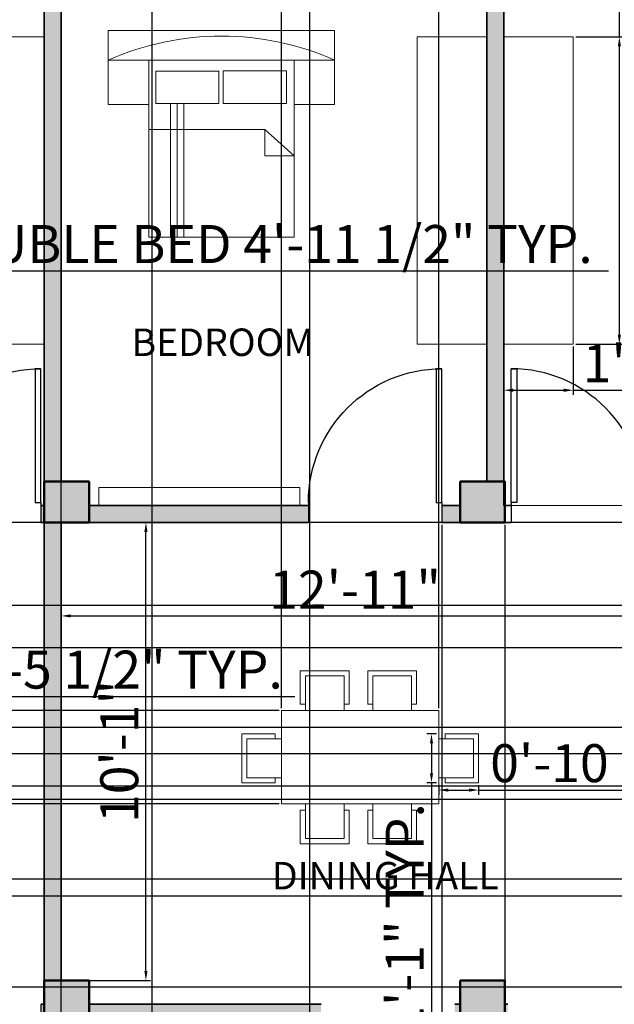
# Model space of a CAD drawing. Units: inches. Extents: x 2312 to 2808, y 1290 to 1909.
# Tile 3 of 5: x 2476 to 2633, y 1503 to 1763. Entities that reach past the tile are written whole.
import ezdxf

# ---------------------------------------------------------------- set-up
doc = ezdxf.new("R2010")
doc.units = ezdxf.units.IN
for name, color, linetype, lineweight in [('A-ANNO-DIMS', 2, 'Continuous', 18), ('A-AREA-IDEN', 7, 'Continuous', 25), ('A-COLS-PATT', 1, 'Continuous', 13), ('A-FLOR-CASE', 181, 'Continuous', 20), ('A-WALL-PATT', 150, 'Continuous', 13), ('COLUMN', 1, 'Continuous', 50), ('DOOR', 50, 'Continuous', 25), ('FUR', 130, 'Continuous', 18), ('WALL', 7, 'Continuous', 35)]:
    doc.layers.add(name, color=color, linetype=linetype, lineweight=lineweight)
doc.styles.get("Standard").update_dxf_attribs({"font": 'arial.ttf'})
doc.dimstyles.new('ISO-25', dxfattribs={"dimtxt": 10, "dimasz": 2.5, "dimexe": 1.25, "dimexo": 0.625, "dimtad": 1, "dimdec": 0, "dimlunit": 4, "dimtxsty": 'Standard', "dimcen": 2.5, "dimadec": 0, "dimazin": 0, "dimtfac": 1, "dimtdec": 0, "dimtmove": 0, "dimatfit": 3, "dimfxl": 1, "dimarcsym": 0})

# ---------------------------------------------------------------- blocks, each defined once
blk = doc.blocks.new('*U2')
for p, q in [((0, 0), (0, -6)), ((40, 0), (40, -6))]:
    blk.add_line(p, q)
blk.add_lwpolyline([(0, 0), (0, 40), (1.75, 40), (1.75, 0)], close=True)
blk.add_arc((0, 0), 40, 0, 90)
blk = doc.blocks.new('*D12')
at = {"layer": 'A-ANNO-DIMS', "color": 0, "lineweight": -2, "transparency": 16777216}
for p, q in [((2604.24, 1764.94), (2740.72, 1765.28)), ((2739.79, 1637.55), (2739.48, 1762.78)), ((2604.56, 1634.72), (2741.04, 1635.06))]:
    blk.add_line(p, q, dxfattribs=at)
at = {"layer": 'A-ANNO-DIMS', "color": 0, "transparency": 16777216}
for points in [[(2739.89, 1762.78), (2739.06, 1762.78), (2739.47, 1765.28)], [(2740.2, 1637.56), (2739.37, 1637.55), (2739.79, 1635.05)]]:
    blk.add_solid(points, dxfattribs=at)
at = {"layer": 'Defpoints', "color": 0, "transparency": 16777216}
for p in [(2603.61, 1764.94), (2739.47, 1765.28), (2603.93, 1634.72)]:
    blk.add_point(p, dxfattribs=at)
at = {"layer": 'A-ANNO-DIMS', "color": 0, "transparency": 16777216, "insert": (2745.36, 1700.18), "char_height": 10, "attachment_point": 5, "rotation": 270.1423}
blk.add_mtext('10\'-10"', dxfattribs=at)
blk = doc.blocks.new('*D22')
at = {"layer": 'A-ANNO-DIMS', "color": 0, "lineweight": -2, "transparency": 16777216}
for p, q in [((2486.93, 1629.59), (2486.93, 1604.33)), ((2641.91, 1629.59), (2641.91, 1604.33)), ((2489.43, 1605.58), (2639.41, 1605.58))]:
    blk.add_line(p, q, dxfattribs=at)
at = {"layer": 'A-ANNO-DIMS', "color": 0, "transparency": 16777216}
for points in [[(2489.43, 1606), (2489.43, 1605.17), (2486.93, 1605.58)], [(2639.41, 1606), (2639.41, 1605.17), (2641.91, 1605.58)]]:
    blk.add_solid(points, dxfattribs=at)
at = {"layer": 'Defpoints', "color": 0, "transparency": 16777216}
for p in [(2486.93, 1630.22), (2641.91, 1630.22), (2641.91, 1605.58)]:
    blk.add_point(p, dxfattribs=at)
at = {"layer": 'A-ANNO-DIMS', "color": 0, "transparency": 16777216, "insert": (2564.42, 1611.23), "char_height": 10, "attachment_point": 5}
blk.add_mtext('12\'-11"', dxfattribs=at)
blk = doc.blocks.new('*D23')
at = {"layer": 'A-ANNO-DIMS', "color": 0, "lineweight": -2, "transparency": 16777216}
for p, q in [((2487.56, 1630.22), (2510.52, 1630.22)), ((2509.27, 1511.99), (2509.27, 1627.72)), ((2487.56, 1509.49), (2510.52, 1509.49))]:
    blk.add_line(p, q, dxfattribs=at)
at = {"layer": 'A-ANNO-DIMS', "color": 0, "transparency": 16777216}
for points in [[(2508.85, 1627.72), (2509.69, 1627.72), (2509.27, 1630.22)], [(2508.85, 1511.99), (2509.69, 1511.99), (2509.27, 1509.49)]]:
    blk.add_solid(points, dxfattribs=at)
at = {"layer": 'Defpoints', "color": 0, "transparency": 16777216}
for p in [(2486.93, 1630.22), (2509.27, 1630.22), (2486.93, 1509.49)]:
    blk.add_point(p, dxfattribs=at)
at = {"layer": 'A-ANNO-DIMS', "color": 0, "transparency": 16777216, "insert": (2503.54, 1569.86), "char_height": 10, "attachment_point": 5, "rotation": 90}
blk.add_mtext('10\'-1"', dxfattribs=at)
blk = doc.blocks.new('BED-DOUBLE')
for p, q in [((0, 46.6), (0, 54.42)), ((0, 54.42), (59.67, 54.42)), ((59.67, 54.42), (59.67, 46.6)), ((16.43, 35.15), (16.43, 0)), ((18.15, 35.15), (18.15, 0)), ((19.9, 35.15), (19.9, 0)), ((10.68, 28.37), (10.68, 28.37)), ((10.68, 28.37), (41.23, 28.37)), ((41.23, 28.37), (41.23, 21.43)), ((48.99, 21.43), (41.23, 28.37)), ((41.23, 21.43), (48.99, 21.43))]:
    blk.add_line(p, q)
for points in [[(10.68, 46.6), (0, 46.6), (0, 34.89), (10.68, 34.89)], [(10.68, 46.6), (48.99, 46.6), (48.99, 0), (10.68, 0)], [(59.67, 46.6), (48.99, 46.6), (48.99, 34.89), (59.67, 34.89)], [(12.51, 43.74), (29.18, 43.74), (29.18, 35.15), (12.51, 35.15)], [(30.28, 43.78), (46.95, 43.78), (46.95, 35.19), (30.28, 35.19)]]:
    blk.add_lwpolyline(points, close=True)
blk.add_arc((29.84, -20.26), 73.22, 65.9516, 114.0484)
blk = doc.blocks.new('CHAIR-DINING')
for p, q in [((0, 1.67), (0, 10.49)), ((0, 10.49), (12.88, 10.49)), ((12.88, 10.49), (12.88, 1.67)), ((1.34, 1.67), (0, 1.67)), ((12.88, 1.67), (11.58, 1.67))]:
    blk.add_line(p, q)
blk.add_lwpolyline([(1.34, 0), (11.58, 0), (11.58, 9.15), (1.34, 9.15)], close=True)
blk = doc.blocks.new('BEDROOM-STORAGE')
blk.add_lwpolyline([(18.34, 80.97), (0, 80.97), (0, 0), (18.34, 0)], close=True)
blk = doc.blocks.new('BEDROOM-WALL-UNIT')
blk.add_lwpolyline([(0, 0), (52.94, 0), (52.94, 4.76), (0, 4.76)], close=True)
blk = doc.blocks.new('*D29')
at = {"layer": 'A-ANNO-DIMS', "color": 0, "lineweight": -2, "transparency": 16777216}
for p, q in [((2382.33, 1704.84), (2382.33, 1695.26)), ((2442, 1704.84), (2442, 1695.26)), ((2384.83, 1696.51), (2439.5, 1696.51)), ((2442, 1696.51), (2631.22, 1696.51))]:
    blk.add_line(p, q, dxfattribs=at)
at = {"layer": 'A-ANNO-DIMS', "color": 0, "transparency": 16777216}
for points in [[(2384.83, 1696.93), (2384.83, 1696.09), (2382.33, 1696.51)], [(2439.5, 1696.93), (2439.5, 1696.09), (2442, 1696.51)]]:
    blk.add_solid(points, dxfattribs=at)
at = {"layer": 'Defpoints', "color": 0, "transparency": 16777216}
for p in [(2382.33, 1705.46), (2442, 1705.46), (2442, 1696.51)]:
    blk.add_point(p, dxfattribs=at)
at = {"layer": 'A-ANNO-DIMS', "color": 0, "transparency": 16777216, "insert": (2537.86, 1702.31), "char_height": 10, "attachment_point": 5}
blk.add_mtext('DOUBLE BED 4\'-11 1/2" TYP.', dxfattribs=at)
blk = doc.blocks.new('*D31')
at = {"layer": 'A-ANNO-DIMS', "color": 0, "lineweight": -2, "transparency": 16777216}
for p, q in [((2634.1, 1758.19), (2634.1, 1909.46)), ((2622.58, 1758.19), (2635.35, 1758.19)), ((2634.1, 1679.72), (2634.1, 1755.69)), ((2622.58, 1677.22), (2635.35, 1677.22))]:
    blk.add_line(p, q, dxfattribs=at)
at = {"layer": 'A-ANNO-DIMS', "color": 0, "transparency": 16777216}
for points in [[(2633.68, 1755.69), (2634.51, 1755.69), (2634.1, 1758.19)], [(2633.68, 1679.72), (2634.51, 1679.72), (2634.1, 1677.22)]]:
    blk.add_solid(points, dxfattribs=at)
at = {"layer": 'Defpoints', "color": 0, "transparency": 16777216}
for p in [(2621.95, 1758.19), (2634.1, 1758.19), (2621.95, 1677.22)]:
    blk.add_point(p, dxfattribs=at)
at = {"layer": 'A-ANNO-DIMS', "color": 0, "transparency": 16777216, "insert": (2628.3, 1835.07), "char_height": 10, "attachment_point": 5, "rotation": 90}
blk.add_mtext('WARDROBE 6\'-9" TYP.', dxfattribs=at)
blk = doc.blocks.new('*D32')
at = {"layer": 'A-ANNO-DIMS', "color": 0, "lineweight": -2, "transparency": 16777216}
for p, q in [((2603.61, 1676.59), (2603.61, 1663.82)), ((2621.95, 1676.59), (2621.95, 1663.82)), ((2606.11, 1665.07), (2619.45, 1665.07)), ((2621.95, 1665.07), (2709.02, 1665.07))]:
    blk.add_line(p, q, dxfattribs=at)
at = {"layer": 'A-ANNO-DIMS', "color": 0, "transparency": 16777216}
for points in [[(2606.11, 1665.49), (2606.11, 1664.65), (2603.61, 1665.07)], [(2619.45, 1665.49), (2619.45, 1664.65), (2621.95, 1665.07)]]:
    blk.add_solid(points, dxfattribs=at)
at = {"layer": 'Defpoints', "color": 0, "transparency": 16777216}
for p in [(2603.61, 1677.22), (2621.95, 1677.22), (2621.95, 1665.07)]:
    blk.add_point(p, dxfattribs=at)
at = {"layer": 'A-ANNO-DIMS', "color": 0, "transparency": 16777216, "insert": (2666.73, 1670.87), "char_height": 10, "attachment_point": 5}
blk.add_mtext('1\'-6 1/2" TYP.', dxfattribs=at)
blk = doc.blocks.new('*D33')
at = {"layer": 'A-ANNO-DIMS', "color": 0, "lineweight": -2, "transparency": 16777216}
for p, q in [((2381.24, 1493.33), (2381.24, 1484.77)), ((2434.18, 1493.33), (2434.18, 1484.77)), ((2383.74, 1486.02), (2431.68, 1486.02)), ((2434.18, 1486.02), (2577.69, 1486.02))]:
    blk.add_line(p, q, dxfattribs=at)
at = {"layer": 'A-ANNO-DIMS', "color": 0, "transparency": 16777216}
for points in [[(2383.74, 1486.43), (2383.74, 1485.6), (2381.24, 1486.02)], [(2431.68, 1486.43), (2431.68, 1485.6), (2434.18, 1486.02)]]:
    blk.add_solid(points, dxfattribs=at)
at = {"layer": 'Defpoints', "color": 0, "transparency": 16777216}
for p in [(2381.24, 1493.96), (2434.18, 1493.96), (2434.18, 1486.02)]:
    blk.add_point(p, dxfattribs=at)
at = {"layer": 'A-ANNO-DIMS', "color": 0, "transparency": 16777216, "insert": (2507.19, 1491.73), "char_height": 10, "attachment_point": 5}
blk.add_mtext('WALL UNIT 4\'-5" TYP.', dxfattribs=at)
blk = doc.blocks.new('*D35')
at = {"layer": 'A-ANNO-DIMS', "color": 0, "lineweight": -2, "transparency": 16777216}
for p, q in [((2585.87, 1574.5), (2583.31, 1574.5)), ((2584.56, 1572), (2584.56, 1564.12)), ((2585.87, 1561.62), (2583.31, 1561.62)), ((2584.56, 1561.62), (2584.56, 1449.68))]:
    blk.add_line(p, q, dxfattribs=at)
at = {"layer": 'A-ANNO-DIMS', "color": 0, "transparency": 16777216}
for points in [[(2584.15, 1572), (2584.98, 1572), (2584.56, 1574.5)], [(2584.15, 1564.12), (2584.98, 1564.12), (2584.56, 1561.62)]]:
    blk.add_solid(points, dxfattribs=at)
at = {"layer": 'Defpoints', "color": 0, "transparency": 16777216}
for p in [(2586.49, 1574.5), (2584.56, 1561.62), (2586.49, 1561.62)]:
    blk.add_point(p, dxfattribs=at)
at = {"layer": 'A-ANNO-DIMS', "color": 0, "transparency": 16777216, "insert": (2578.77, 1504.4), "char_height": 10, "attachment_point": 5, "rotation": 90}
blk.add_mtext('CHAIR 1\'-1" TYP.', dxfattribs=at)
blk = doc.blocks.new('*D36')
at = {"layer": 'A-ANNO-DIMS', "color": 0, "lineweight": -2, "transparency": 16777216}
for p, q in [((2586.49, 1560.99), (2586.49, 1558.44)), ((2596.99, 1560.99), (2596.99, 1558.44)), ((2588.99, 1559.69), (2594.49, 1559.69)), ((2596.99, 1559.69), (2692.76, 1559.69))]:
    blk.add_line(p, q, dxfattribs=at)
at = {"layer": 'A-ANNO-DIMS', "color": 0, "transparency": 16777216}
for points in [[(2588.99, 1560.1), (2588.99, 1559.27), (2586.49, 1559.69)], [(2594.49, 1560.1), (2594.49, 1559.27), (2596.99, 1559.69)]]:
    blk.add_solid(points, dxfattribs=at)
at = {"layer": 'Defpoints', "color": 0, "transparency": 16777216}
for p in [(2586.49, 1561.62), (2596.99, 1561.62), (2596.99, 1559.69)]:
    blk.add_point(p, dxfattribs=at)
at = {"layer": 'A-ANNO-DIMS', "color": 0, "transparency": 16777216, "insert": (2646.12, 1565.48), "char_height": 10, "attachment_point": 5}
blk.add_mtext('0\'-10 1/2" TYP.', dxfattribs=at)
blk = doc.blocks.new('*D37')
at = {"layer": 'A-ANNO-DIMS', "color": 0, "lineweight": -2, "transparency": 16777216}
for p, q in [((2380.65, 1586.33), (2380.65, 1583.1)), ((2398.06, 1586.33), (2398.06, 1583.1)), ((2383.15, 1584.35), (2395.56, 1584.35)), ((2398.06, 1584.35), (2548.49, 1584.35))]:
    blk.add_line(p, q, dxfattribs=at)
at = {"layer": 'A-ANNO-DIMS', "color": 0, "transparency": 16777216}
for points in [[(2383.15, 1584.76), (2383.15, 1583.93), (2380.65, 1584.35)], [(2395.56, 1584.76), (2395.56, 1583.93), (2398.06, 1584.35)]]:
    blk.add_solid(points, dxfattribs=at)
at = {"layer": 'Defpoints', "color": 0, "transparency": 16777216}
for p in [(2380.65, 1586.96), (2398.06, 1586.96), (2398.06, 1584.35)]:
    blk.add_point(p, dxfattribs=at)
at = {"layer": 'A-ANNO-DIMS', "color": 0, "transparency": 16777216, "insert": (2474.53, 1590.14), "char_height": 10, "attachment_point": 5}
blk.add_mtext('BURNER 1\'-5 1/2" TYP.', dxfattribs=at)
blk = doc.blocks.new('*D41')
at = {"layer": 'A-ANNO-DIMS', "color": 0, "lineweight": -2, "transparency": 16777216}
for p, q in [((2443.93, 1546.83), (2443.93, 1804.57)), ((2482.43, 1510.12), (2482.43, 1804.57)), ((2446.43, 1803.32), (2479.93, 1803.32)), ((2482.43, 1803.32), (2536.06, 1803.32))]:
    blk.add_line(p, q, dxfattribs=at)
at = {"layer": 'A-ANNO-DIMS', "color": 0, "transparency": 16777216}
for points in [[(2446.43, 1803.73), (2446.43, 1802.9), (2443.93, 1803.32)], [(2479.93, 1803.73), (2479.93, 1802.9), (2482.43, 1803.32)]]:
    blk.add_solid(points, dxfattribs=at)
at = {"layer": 'Defpoints', "color": 0, "transparency": 16777216}
for p in [(2482.43, 1803.32), (2443.93, 1546.2), (2482.43, 1509.49)]:
    blk.add_point(p, dxfattribs=at)
at = {"layer": 'A-ANNO-DIMS', "color": 0, "transparency": 16777216, "insert": (2510.5, 1809.12), "char_height": 10, "attachment_point": 5}
blk.add_mtext('3\'-2 1/2"', dxfattribs=at)
blk = doc.blocks.new('*D43')
at = {"layer": 'A-ANNO-DIMS', "color": 0, "lineweight": -2, "transparency": 16777216}
for p, q in [((2486.93, 1401.34), (2486.93, 1804.57)), ((2510.93, 1401.34), (2510.93, 1804.57)), ((2489.43, 1803.32), (2508.43, 1803.32)), ((2510.93, 1803.32), (2541.44, 1803.32))]:
    blk.add_line(p, q, dxfattribs=at)
at = {"layer": 'A-ANNO-DIMS', "color": 0, "transparency": 16777216}
for points in [[(2489.43, 1803.73), (2489.43, 1802.9), (2486.93, 1803.32)], [(2508.43, 1803.73), (2508.43, 1802.9), (2510.93, 1803.32)]]:
    blk.add_solid(points, dxfattribs=at)
at = {"layer": 'Defpoints', "color": 0, "transparency": 16777216}
for p in [(2510.93, 1803.32), (2486.93, 1400.72), (2510.93, 1400.72)]:
    blk.add_point(p, dxfattribs=at)
at = {"layer": 'A-ANNO-DIMS', "color": 0, "transparency": 16777216, "insert": (2527.44, 1809.05), "char_height": 10, "attachment_point": 5}
blk.add_mtext('2\'-0"', dxfattribs=at)
blk = doc.blocks.new('*D50')
at = {"layer": 'A-ANNO-DIMS', "color": 0, "lineweight": -2, "transparency": 16777216}
for p, q in [((2446.36, 1635.34), (2446.36, 1804.57)), ((2482.43, 1635.34), (2482.43, 1804.57)), ((2448.86, 1803.32), (2479.93, 1803.32))]:
    blk.add_line(p, q, dxfattribs=at)
at = {"layer": 'A-ANNO-DIMS', "color": 0, "transparency": 16777216}
for points in [[(2448.86, 1803.73), (2448.86, 1802.9), (2446.36, 1803.32)], [(2479.93, 1803.73), (2479.93, 1802.9), (2482.43, 1803.32)]]:
    blk.add_solid(points, dxfattribs=at)
at = {"layer": 'Defpoints', "color": 0, "transparency": 16777216}
for p in [(2482.43, 1803.32), (2446.36, 1634.72), (2482.43, 1634.72)]:
    blk.add_point(p, dxfattribs=at)
at = {"layer": 'A-ANNO-DIMS', "color": 0, "transparency": 16777216, "insert": (2464.4, 1809.05), "char_height": 10, "attachment_point": 5}
blk.add_mtext('3\'-0"', dxfattribs=at)
blk = doc.blocks.new('*D54')
at = {"layer": 'A-ANNO-DIMS', "color": 0, "lineweight": -2, "transparency": 16777216}
for p, q in [((2545.01, 1581.25), (2545.01, 1804.57)), ((2586.49, 1581.25), (2586.49, 1804.57)), ((2547.51, 1803.32), (2583.99, 1803.32)), ((2586.49, 1803.32), (2640.12, 1803.32))]:
    blk.add_line(p, q, dxfattribs=at)
at = {"layer": 'A-ANNO-DIMS', "color": 0, "transparency": 16777216}
for points in [[(2547.51, 1803.73), (2547.51, 1802.9), (2545.01, 1803.32)], [(2583.99, 1803.73), (2583.99, 1802.9), (2586.49, 1803.32)]]:
    blk.add_solid(points, dxfattribs=at)
at = {"layer": 'Defpoints', "color": 0, "transparency": 16777216}
for p in [(2586.49, 1803.32), (2545.01, 1580.62), (2586.49, 1580.62)]:
    blk.add_point(p, dxfattribs=at)
at = {"layer": 'A-ANNO-DIMS', "color": 0, "transparency": 16777216, "insert": (2614.56, 1809.12), "char_height": 10, "attachment_point": 5}
blk.add_mtext('3\'-5 1/2"', dxfattribs=at)
blk = doc.blocks.new('*D55')
at = {"layer": 'A-ANNO-DIMS', "color": 0, "lineweight": -2, "transparency": 16777216}
for p, q in [((2332.83, 1580.62), (2332.83, 1634.43)), ((2544.39, 1580.62), (2331.58, 1580.62)), ((2332.83, 1558.54), (2332.83, 1578.12)), ((2544.39, 1556.04), (2331.58, 1556.04))]:
    blk.add_line(p, q, dxfattribs=at)
at = {"layer": 'A-ANNO-DIMS', "color": 0, "transparency": 16777216}
for points in [[(2332.42, 1578.12), (2333.25, 1578.12), (2332.83, 1580.62)], [(2332.42, 1558.54), (2333.25, 1558.54), (2332.83, 1556.04)]]:
    blk.add_solid(points, dxfattribs=at)
at = {"layer": 'Defpoints', "color": 0, "transparency": 16777216}
for p in [(2332.83, 1580.62), (2545.01, 1580.62), (2545.01, 1556.04)]:
    blk.add_point(p, dxfattribs=at)
at = {"layer": 'A-ANNO-DIMS', "color": 0, "transparency": 16777216, "insert": (2327.04, 1608.77), "char_height": 10, "attachment_point": 5, "rotation": 90}
blk.add_mtext('2\'-0 1/2"', dxfattribs=at)
blk = doc.blocks.new('*D63')
at = {"layer": 'A-ANNO-DIMS', "color": 0, "lineweight": -2, "transparency": 16777216}
for p, q in [((2799.03, 1531.79), (2799.03, 1562.3)), ((2433.46, 1531.79), (2800.28, 1531.79)), ((2799.03, 1510.3), (2799.03, 1529.29)), ((2433.46, 1507.8), (2800.28, 1507.8))]:
    blk.add_line(p, q, dxfattribs=at)
at = {"layer": 'A-ANNO-DIMS', "color": 0, "transparency": 16777216}
for points in [[(2798.62, 1529.29), (2799.45, 1529.29), (2799.03, 1531.79)], [(2798.62, 1510.3), (2799.45, 1510.3), (2799.03, 1507.8)]]:
    blk.add_solid(points, dxfattribs=at)
at = {"layer": 'Defpoints', "color": 0, "transparency": 16777216}
for p in [(2432.83, 1531.79), (2799.03, 1531.79), (2432.83, 1507.8)]:
    blk.add_point(p, dxfattribs=at)
at = {"layer": 'A-ANNO-DIMS', "color": 0, "transparency": 16777216, "insert": (2793.3, 1548.3), "char_height": 10, "attachment_point": 5, "rotation": 90}
blk.add_mtext('2\'-0"', dxfattribs=at)
blk = doc.blocks.new('*D65')
at = {"layer": 'A-ANNO-DIMS', "color": 0, "lineweight": -2, "transparency": 16777216}
for p, q in [((2710.81, 1557.21), (2331.58, 1557.21)), ((2332.83, 1554.71), (2332.83, 1538.71)), ((2710.81, 1536.21), (2331.58, 1536.21)), ((2332.83, 1536.21), (2332.83, 1506.82))]:
    blk.add_line(p, q, dxfattribs=at)
at = {"layer": 'A-ANNO-DIMS', "color": 0, "transparency": 16777216}
for points in [[(2332.42, 1554.71), (2333.25, 1554.71), (2332.83, 1557.21)], [(2332.42, 1538.71), (2333.25, 1538.71), (2332.83, 1536.21)]]:
    blk.add_solid(points, dxfattribs=at)
at = {"layer": 'Defpoints', "color": 0, "transparency": 16777216}
for p in [(2711.43, 1557.21), (2332.83, 1536.21), (2711.43, 1536.21)]:
    blk.add_point(p, dxfattribs=at)
at = {"layer": 'A-ANNO-DIMS', "color": 0, "transparency": 16777216, "insert": (2327.1, 1520.27), "char_height": 10, "attachment_point": 5, "rotation": 90}
blk.add_mtext('1\'-9"', dxfattribs=at)
blk = doc.blocks.new('*D67')
at = {"layer": 'A-ANNO-DIMS', "color": 0, "lineweight": -2, "transparency": 16777216}
for p, q in [((2486.93, 1499.34), (2486.93, 1804.57)), ((2552.51, 1499.34), (2552.51, 1804.57)), ((2489.43, 1803.32), (2550.01, 1803.32))]:
    blk.add_line(p, q, dxfattribs=at)
at = {"layer": 'A-ANNO-DIMS', "color": 0, "transparency": 16777216}
for points in [[(2489.43, 1803.73), (2489.43, 1802.9), (2486.93, 1803.32)], [(2550.01, 1803.73), (2550.01, 1802.9), (2552.51, 1803.32)]]:
    blk.add_solid(points, dxfattribs=at)
at = {"layer": 'Defpoints', "color": 0, "transparency": 16777216}
for p in [(2552.51, 1803.32), (2486.93, 1498.72), (2552.51, 1498.72)]:
    blk.add_point(p, dxfattribs=at)
at = {"layer": 'A-ANNO-DIMS', "color": 0, "transparency": 16777216, "insert": (2519.72, 1809.11), "char_height": 10, "attachment_point": 5}
blk.add_mtext('5\'-5 1/2"', dxfattribs=at)
blk = doc.blocks.new('*D71')
at = {"layer": 'A-ANNO-DIMS', "color": 0, "lineweight": -2, "transparency": 16777216}
for p, q in [((2587.32, 1629.59), (2587.32, 1326.46)), ((2603.93, 1629.59), (2603.93, 1326.46)), ((2589.82, 1327.71), (2601.43, 1327.71)), ((2603.93, 1327.71), (2656.63, 1327.71))]:
    blk.add_line(p, q, dxfattribs=at)
at = {"layer": 'A-ANNO-DIMS', "color": 0, "transparency": 16777216}
for points in [[(2589.82, 1328.13), (2589.82, 1327.3), (2587.32, 1327.71)], [(2601.43, 1328.13), (2601.43, 1327.3), (2603.93, 1327.71)]]:
    blk.add_solid(points, dxfattribs=at)
at = {"layer": 'Defpoints', "color": 0, "transparency": 16777216}
for p in [(2587.32, 1630.22), (2603.93, 1630.22), (2603.93, 1327.71)]:
    blk.add_point(p, dxfattribs=at)
at = {"layer": 'A-ANNO-DIMS', "color": 0, "transparency": 16777216, "insert": (2631.53, 1333.51), "char_height": 10, "attachment_point": 5}
blk.add_mtext('1\'-4 1/2"', dxfattribs=at)
blk = doc.blocks.new('*D72')
at = {"layer": 'A-ANNO-DIMS', "color": 0, "lineweight": -2, "transparency": 16777216}
for p, q in [((2702.81, 1576.18), (2331.58, 1576.18)), ((2332.83, 1573.68), (2332.83, 1571.72)), ((2710.81, 1569.22), (2331.58, 1569.22)), ((2332.83, 1569.22), (2332.83, 1538.88))]:
    blk.add_line(p, q, dxfattribs=at)
at = {"layer": 'A-ANNO-DIMS', "color": 0, "transparency": 16777216}
for points in [[(2332.42, 1573.68), (2333.25, 1573.68), (2332.83, 1576.18)], [(2332.42, 1571.72), (2333.25, 1571.72), (2332.83, 1569.22)]]:
    blk.add_solid(points, dxfattribs=at)
at = {"layer": 'Defpoints', "color": 0, "transparency": 16777216}
for p in [(2703.43, 1576.18), (2332.83, 1569.22), (2711.43, 1569.22)]:
    blk.add_point(p, dxfattribs=at)
at = {"layer": 'A-ANNO-DIMS', "color": 0, "transparency": 16777216, "insert": (2327.1, 1552.8), "char_height": 10, "attachment_point": 5, "rotation": 90}
blk.add_mtext('0\'-7"', dxfattribs=at)
blk = doc.blocks.new('*D74')
at = {"layer": 'A-ANNO-DIMS', "color": 0, "lineweight": -2, "transparency": 16777216}
for p, q in [((2799.03, 1608.44), (2799.03, 1669.84)), ((2403.21, 1608.44), (2800.28, 1608.44)), ((2799.03, 1563.31), (2799.03, 1605.94)), ((2403.21, 1560.81), (2800.28, 1560.81))]:
    blk.add_line(p, q, dxfattribs=at)
at = {"layer": 'A-ANNO-DIMS', "color": 0, "transparency": 16777216}
for points in [[(2798.62, 1605.94), (2799.45, 1605.94), (2799.03, 1608.44)], [(2798.62, 1563.31), (2799.45, 1563.31), (2799.03, 1560.81)]]:
    blk.add_solid(points, dxfattribs=at)
at = {"layer": 'Defpoints', "color": 0, "transparency": 16777216}
for p in [(2402.58, 1608.44), (2799.03, 1608.44), (2402.58, 1560.81)]:
    blk.add_point(p, dxfattribs=at)
at = {"layer": 'A-ANNO-DIMS', "color": 0, "transparency": 16777216, "insert": (2793.24, 1640.39), "char_height": 10, "attachment_point": 5, "rotation": 90}
blk.add_mtext('3\'-11 1/2"', dxfattribs=at)
blk = doc.blocks.new('*D75')
at = {"layer": 'A-ANNO-DIMS', "color": 0, "lineweight": -2, "transparency": 16777216}
for p, q in [((2641.28, 1630.22), (2331.58, 1630.22)), ((2332.83, 1627.72), (2332.83, 1599.71)), ((2641.28, 1597.21), (2331.58, 1597.21))]:
    blk.add_line(p, q, dxfattribs=at)
at = {"layer": 'A-ANNO-DIMS', "color": 0, "transparency": 16777216}
for points in [[(2332.42, 1627.72), (2333.25, 1627.72), (2332.83, 1630.22)], [(2332.42, 1599.71), (2333.25, 1599.71), (2332.83, 1597.21)]]:
    blk.add_solid(points, dxfattribs=at)
at = {"layer": 'Defpoints', "color": 0, "transparency": 16777216}
for p in [(2641.91, 1630.22), (2332.83, 1597.21), (2641.91, 1597.21)]:
    blk.add_point(p, dxfattribs=at)
at = {"layer": 'A-ANNO-DIMS', "color": 0, "transparency": 16777216, "insert": (2327.1, 1613.71), "char_height": 10, "attachment_point": 5, "rotation": 90}
blk.add_mtext('2\'-9"', dxfattribs=at)

msp = doc.modelspace()

# ---------------------------------------------------------------- hatches: boundary and pattern name
at = {"layer": 'A-COLS-PATT'}
h = msp.add_hatch(color=256, dxfattribs=at)
h.dxf.hatch_style = 1
h.paths.add_polyline_path([(2372.28, 1775.72), (2360.43, 1775.72), (2360.43, 1764.94), (2372.28, 1764.94)])
h.paths.add_polyline_path([(2486.97, 1775.72), (2475.12, 1775.72), (2475.12, 1764.94), (2486.93, 1764.94), (2486.93, 1766.72)])
h.paths.add_polyline_path([(2610.92, 1775.72), (2599.07, 1775.72), (2599.07, 1766.72), (2599.11, 1766.72), (2599.11, 1764.94), (2610.92, 1764.94)])
h.paths.add_polyline_path([(2720.43, 1775.72), (2708.59, 1775.72), (2708.59, 1764.94), (2720.43, 1764.94)])
h.paths.add_polyline_path([(2723.28, 1640.11), (2711.43, 1640.11), (2711.43, 1629.34), (2723.28, 1629.34)])
h.paths.add_polyline_path([(2603.61, 1640.99), (2592.09, 1640.99), (2592.09, 1630.22), (2603.93, 1630.22), (2603.93, 1634.72), (2603.61, 1634.72)])
h.paths.add_polyline_path([(2494.28, 1640.99), (2482.43, 1640.99), (2482.43, 1630.22), (2494.28, 1630.22)])
h.paths.add_polyline_path([(2372.28, 1640.99), (2360.43, 1640.99), (2360.43, 1630.22), (2372.28, 1630.22)])
h.paths.add_polyline_path([(2372.28, 1509.49), (2360.43, 1509.49), (2360.43, 1498.72), (2372.28, 1498.72)])
h.paths.add_polyline_path([(2494.28, 1509.49), (2482.43, 1509.49), (2482.43, 1498.72), (2494.28, 1498.72)])
h.paths.add_polyline_path([(2603.93, 1509.49), (2592.09, 1509.49), (2592.09, 1498.72), (2603.93, 1498.72)])
h.paths.add_polyline_path([(2723.28, 1509.26), (2711.43, 1509.26), (2711.43, 1498.48), (2723.28, 1498.48)])
h.paths.add_polyline_path([(2720.43, 1378.49), (2708.59, 1378.49), (2708.59, 1367.72), (2720.43, 1367.72)])
h.paths.add_polyline_path([(2610.2, 1378.49), (2598.36, 1378.49), (2598.36, 1367.72), (2610.2, 1367.72)])
h.paths.add_polyline_path([(2486.94, 1376.72), (2486.93, 1376.72), (2486.93, 1378.49), (2475.1, 1378.49), (2475.1, 1367.72), (2486.94, 1367.72)])
h.paths.add_polyline_path([(2372.28, 1378.49), (2360.43, 1378.49), (2360.43, 1367.72), (2372.28, 1367.72)])
at = {"layer": 'A-WALL-PATT'}
h = msp.add_hatch(color=256, dxfattribs=at)
h.dxf.hatch_style = 1
h.paths.add_polyline_path([(2369.43, 1764.94), (2360.43, 1764.94), (2360.43, 1640.99), (2369.43, 1640.99)])
h.paths.add_polyline_path([(2720.43, 1764.94), (2711.43, 1764.94), (2711.43, 1640.11), (2720.43, 1640.11)])
h.paths.add_polyline_path([(2552.09, 1634.72), (2494.28, 1634.72), (2494.28, 1630.22), (2552.09, 1630.22)])
h.paths.add_polyline_path([(2446.36, 1634.72), (2372.28, 1634.72), (2372.28, 1630.22), (2405.43, 1630.22), (2439.43, 1630.22), (2446.36, 1630.22)])
h.paths.add_polyline_path([(2443.93, 1630.22), (2439.43, 1630.22), (2439.43, 1596.05), (2443.93, 1596.05)])
h.paths.add_polyline_path([(2486.93, 1630.22), (2482.43, 1630.22), (2482.43, 1509.49), (2486.93, 1509.49)])
h.paths.add_polyline_path([(2443.93, 1546.2), (2439.43, 1546.2), (2439.43, 1503.22), (2372.28, 1503.22), (2372.28, 1498.72), (2443.93, 1498.72)])
h.paths.add_polyline_path([(2555.45, 1503.22), (2494.28, 1503.22), (2494.28, 1498.72), (2555.45, 1498.72)])
h.paths.add_polyline_path([(2711.43, 1503.22), (2639.88, 1503.22), (2639.88, 1498.72), (2711.43, 1498.72)])
h.paths.add_polyline_path([(2646.41, 1564.72), (2711.43, 1564.72), (2711.43, 1569.22), (2646.41, 1569.22), (2646.41, 1597.21), (2641.91, 1597.21), (2641.91, 1564.72), (2641.91, 1536.48), (2646.41, 1536.48)])
h.paths.add_polyline_path([(2720.43, 1498.48), (2711.43, 1498.48), (2711.43, 1378.49), (2720.43, 1378.49)])
h.paths.add_polyline_path([(2369.43, 1498.72), (2360.43, 1498.72), (2360.43, 1378.49), (2369.43, 1378.49)])
h.paths.add_polyline_path([(2486.93, 1498.72), (2482.43, 1498.72), (2482.43, 1378.49), (2486.93, 1378.49)])
h.paths.add_polyline_path([(2603.93, 1498.72), (2599.11, 1498.72), (2599.11, 1378.49), (2603.93, 1378.49)])
h.paths.add_polyline_path([(2510.36, 1766.72), (2510.36, 1775.72), (2486.97, 1775.72), (2486.97, 1766.72)])
h.paths.add_polyline_path([(2571.02, 1775.72), (2571.02, 1766.72), (2599.07, 1766.72), (2599.07, 1775.72)])
h.paths.add_polyline_path([(2393.8, 1766.72), (2393.8, 1775.72), (2372.28, 1775.72), (2372.28, 1766.72)])
h.paths.add_polyline_path([(2454.45, 1775.72), (2454.45, 1766.72), (2475.12, 1766.72), (2475.12, 1775.72)])
h.paths.add_polyline_path([(2694.96, 1775.72), (2694.96, 1766.72), (2708.59, 1766.72), (2708.59, 1775.72)])
h.paths.add_polyline_path([(2634.31, 1766.72), (2634.31, 1775.72), (2610.92, 1775.72), (2610.92, 1766.72)])
h.paths.add_polyline_path([(2392.25, 1367.72), (2392.25, 1376.72), (2372.28, 1376.72), (2372.28, 1367.72)])
h.paths.add_polyline_path([(2452.9, 1376.72), (2452.9, 1367.72), (2475.1, 1367.72), (2475.1, 1376.72)])
h.paths.add_polyline_path([(2508.56, 1376.72), (2508.56, 1367.72), (2558.63, 1367.72), (2558.63, 1370.65), (2558.63, 1376.72)])
h.paths.add_polyline_path([(2488.96, 1367.72), (2488.96, 1376.72), (2486.94, 1376.72), (2486.94, 1367.72)])
h.paths.add_polyline_path([(2634.6, 1367.72), (2634.6, 1376.72), (2610.2, 1376.72), (2610.2, 1367.72)])
h.paths.add_polyline_path([(2695.25, 1376.72), (2695.25, 1367.72), (2708.59, 1367.72), (2708.59, 1376.72)])
h.paths.add_polyline_path([(2360.43, 1590.4), (2369.43, 1590.4), (2369.43, 1630.22), (2360.43, 1630.22)])
h.paths.add_polyline_path([(2369.43, 1543.07), (2360.43, 1543.07), (2360.43, 1509.49), (2369.43, 1509.49)])
h.paths.add_polyline_path([(2720.43, 1531.67), (2711.43, 1531.67), (2711.43, 1509.26), (2720.43, 1509.26)])
h.paths.add_polyline_path([(2720.43, 1572.68), (2711.43, 1572.68), (2711.43, 1558.71), (2720.43, 1558.71)])
h.paths.add_polyline_path([(2711.43, 1599.72), (2720.43, 1599.72), (2720.43, 1629.34), (2711.43, 1629.34)])
h = msp.add_hatch(color=256, dxfattribs=at)
h.dxf.hatch_style = 1
h.paths.add_polyline_path([(2486.93, 1764.94), (2482.43, 1764.94), (2482.43, 1640.99), (2486.93, 1640.99)])
h.paths.add_polyline_path([(2603.61, 1764.94), (2599.11, 1764.94), (2599.11, 1640.99), (2603.61, 1640.99)])
h = msp.add_hatch(color=256, dxfattribs=at)
h.dxf.hatch_style = 1
h.paths.add_polyline_path([(2482.43, 1634.72), (2481.59, 1634.72), (2481.59, 1630.22), (2482.43, 1630.22)])
h.paths.add_polyline_path([(2592.09, 1634.72), (2587.32, 1634.72), (2587.32, 1630.22), (2592.09, 1630.22)])
h.paths.add_polyline_path([(2646.41, 1630.22), (2641.91, 1630.22), (2641.91, 1626.81), (2646.41, 1626.81)])
h = msp.add_hatch(color=256, dxfattribs=at)
h.dxf.hatch_style = 1
h.paths.add_polyline_path([(2446.46, 1503.22), (2443.93, 1503.22), (2443.93, 1498.72), (2446.46, 1498.72)])
h.paths.add_polyline_path([(2482.43, 1503.22), (2481.69, 1503.22), (2481.69, 1498.72), (2482.43, 1498.72)])
h.paths.add_polyline_path([(2592.09, 1503.22), (2590.68, 1503.22), (2590.68, 1498.72), (2592.09, 1498.72)])
h.paths.add_polyline_path([(2604.66, 1503.22), (2603.93, 1503.22), (2603.93, 1498.72), (2604.66, 1498.72)])

# ---------------------------------------------------------------- linework, layer by layer
at = {"layer": 'COLUMN'}
for points in [[(2482.43, 1640.99), (2494.28, 1640.99), (2494.28, 1630.22), (2482.43, 1630.22)], [(2592.09, 1640.99), (2603.93, 1640.99), (2603.93, 1630.22), (2592.09, 1630.22)], [(2482.43, 1509.49), (2494.28, 1509.49), (2494.28, 1498.72), (2482.43, 1498.72)], [(2592.09, 1509.49), (2603.93, 1509.49), (2603.93, 1498.72), (2592.09, 1498.72)]]:
    msp.add_lwpolyline(points, close=True, dxfattribs=at)
at = {"layer": 'FUR'}
for p, q in [((2551.32, 1582.3), (2551.32, 1582.3)), ((2569.09, 1582.3), (2569.09, 1582.3)), ((2588.17, 1573.15), (2588.17, 1573.15))]:
    msp.add_line(p, q, dxfattribs=at)
msp.add_lwpolyline([(2545.01, 1580.62), (2586.49, 1580.62), (2586.49, 1556.04), (2545.01, 1556.04)], close=True, dxfattribs=at)
at = {"layer": 'WALL'}
for p, q in [((2482.43, 1764.94), (2482.43, 1634.72)), ((2486.93, 1766.72), (2486.93, 1640.99)), ((2599.11, 1766.72), (2599.11, 1640.99)), ((2603.61, 1764.94), (2603.61, 1634.72)), ((2482.43, 1634.72), (2481.59, 1634.72)), ((2482.43, 1634.72), (2482.43, 1378.49)), ((2552.09, 1634.72), (2494.28, 1634.72)), ((2592.09, 1634.72), (2587.32, 1634.72)), ((2603.93, 1634.72), (2603.61, 1634.72)), ((2603.61, 1634.72), (2605.53, 1634.72)), ((2603.93, 1634.72), (2603.93, 1630.22)), ((2486.93, 1630.22), (2481.59, 1630.22)), ((2486.93, 1630.22), (2486.93, 1509.49)), ((2552.09, 1630.22), (2486.93, 1630.22)), ((2605.53, 1630.22), (2587.32, 1630.22)), ((2481.69, 1503.22), (2482.43, 1503.22)), ((2494.28, 1503.22), (2555.45, 1503.22)), ((2590.68, 1503.22), (2592.09, 1503.22)), ((2603.93, 1503.22), (2603.93, 1378.49)), ((2603.93, 1503.22), (2604.66, 1503.22))]:
    msp.add_line(p, q, dxfattribs=at)

# ---------------------------------------------------------------- block references
at = {"layer": 'A-FLOR-CASE'}
for name, p in [('BEDROOM-STORAGE', (2464.09, 1677.22)), ('BEDROOM-STORAGE', (2580.77, 1677.22)), ('BEDROOM-STORAGE', (2603.61, 1677.22)), ('BEDROOM-WALL-UNIT', (2496.89, 1634.72))]:
    msp.add_blockref(name, p, dxfattribs=at)
at = {"layer": 'DOOR', "yscale": 0.8806546932443936, "zscale": 0.8806546932443936}
for p, xscale in [((2481.59, 1635.5), -0.8806546932443936), ((2587.32, 1635.5), -0.8806546932443936), ((2605.53, 1635.5), 0.8806546932443936)]:
    msp.add_blockref('*U2', p, dxfattribs=dict(at, xscale=xscale))
at = {"layer": 'DOOR', "xscale": 0.8806546932443936, "yscale": 0.8806546932443936, "zscale": 0.8806546932443936, "rotation": 180}
msp.add_blockref('*U2', (2481.69, 1497.93), dxfattribs=at)
at = {"layer": 'FUR'}
for name, p in [('BED-DOUBLE', (2499.35, 1705.46)), ('CHAIR-DINING', (2549.98, 1580.62)), ('CHAIR-DINING', (2567.75, 1580.62))]:
    msp.add_blockref(name, p, dxfattribs=at)
at = {"layer": 'FUR', "extrusion": (0, 0, -1), "zscale": -1}
for p, rotation in [((-2545.01, 1574.49), 270.0000000000029), ((-2549.98, 1556.04), 180), ((-2567.75, 1556.04), 180)]:
    msp.add_blockref('CHAIR-DINING', p, dxfattribs=dict(at, rotation=rotation))
at = {"layer": 'FUR', "rotation": 270.000000000007}
msp.add_blockref('CHAIR-DINING', (2586.49, 1574.49), dxfattribs=at)

# ---------------------------------------------------------------- texts
at = {"layer": 'A-AREA-IDEN', "attachment_point": 1}
for s, insert, char_height in [('BEDROOM', (2505.48, 1681.34), 7.244), ('DINING HALL', (2542.48, 1540.74), 7.2437)]:
    msp.add_mtext_dynamic_manual_height_columns(s, width=196.5617, gutter_width=36.22, heights=[0], dxfattribs=dict(at, insert=insert, char_height=char_height))

# ---------------------------------------------------------------- dimensions: what is measured, and where the dimension line sits
at = {"layer": 'A-ANNO-DIMS'}
for base, p1, p2, angle, text, picture, middle in [((2634.1, 1758.19), (2621.95, 1677.22), (2621.95, 1758.19), 90, 'WARDROBE <> TYP.', '*D31', (2628.3, 1835.07)), ((2596.99, 1559.69), (2586.49, 1561.62), (2596.99, 1561.62), 0, '<> TYP.', '*D36', (2646.12, 1565.48)), ((2584.56, 1561.62), (2586.49, 1574.5), (2586.49, 1561.62), 270, 'CHAIR <> TYP.', '*D35', (2578.77, 1504.4))]:
    dim = msp.add_linear_dim(base=base, p1=p1, p2=p2, angle=angle, text=text, dimstyle='ISO-25', override={"dimdec": 1, "dimlfac": 1, "dimrnd": 0, "dimzin": 1, "dimdsep": 46, "dimlunit": 4, "dimfrac": 2}, dxfattribs=at)
    dim.commit()
    dim.dimension.update_dxf_attribs({"geometry": picture, "text_midpoint": middle})
for base, p1, p2, override, picture, middle in [((2482.43, 1803.32), (2443.93, 1546.2), (2482.43, 1509.49), {"dimdec": 1, "dimlfac": 1, "dimrnd": 0, "dimzin": 1, "dimdsep": 46, "dimlunit": 4, "dimfrac": 2}, '*D41', (2510.5, 1809.12)), ((2552.51, 1803.32), (2486.93, 1498.72), (2552.51, 1498.72), {"dimdec": 1, "dimlfac": 1, "dimrnd": 0, "dimzin": 1, "dimdsep": 46, "dimlunit": 4, "dimfrac": 2}, '*D67', (2519.72, 1809.11)), ((2586.49, 1803.32), (2545.01, 1580.62), (2586.49, 1580.62), {"dimdec": 1, "dimlfac": 1, "dimrnd": 0, "dimzin": 1, "dimdsep": 46, "dimlunit": 4, "dimfrac": 2}, '*D54', (2614.56, 1809.12)), ((2482.43, 1803.32), (2446.36, 1634.72), (2482.43, 1634.72), {"dimdec": 1, "dimlfac": 1, "dimrnd": 0, "dimzin": 1, "dimdsep": 46, "dimlunit": 4, "dimfrac": 2}, '*D50', (2464.4, 1809.05)), ((2510.93, 1803.32), (2486.93, 1400.72), (2510.93, 1400.72), {"dimdec": 1, "dimlfac": 1, "dimrnd": 0, "dimzin": 1, "dimdsep": 46, "dimlunit": 4, "dimfrac": 2}, '*D43', (2527.44, 1809.05)), ((2641.91, 1605.58), (2486.93, 1630.22), (2641.91, 1630.22), {"dimclrd": 0, "dimclre": 0, "dimclrt": 0}, '*D22', (2564.42, 1611.23)), ((2603.93, 1327.71), (2587.32, 1630.22), (2603.93, 1630.22), {"dimdec": 1, "dimlfac": 1, "dimrnd": 0, "dimzin": 1, "dimdsep": 46, "dimlunit": 4, "dimfrac": 2}, '*D71', (2631.53, 1333.51))]:
    dim = msp.add_linear_dim(base=base, p1=p1, p2=p2, dimstyle='ISO-25', override=override, dxfattribs=at)
    dim.commit()
    dim.dimension.update_dxf_attribs({"geometry": picture, "text_midpoint": middle})
dim = msp.add_aligned_dim(p1=(2603.93, 1634.72), p2=(2603.61, 1764.94), distance=-135.86, dimstyle='ISO-25', override={"dimclrd": 0, "dimclre": 0, "dimclrt": 0}, dxfattribs=at)
dim.commit()
dim.dimension.update_dxf_attribs({"geometry": '*D12', "text_midpoint": (2745.36, 1700.18)})
for base, p1, p2, text, picture, middle in [((2442, 1696.51), (2382.33, 1705.46), (2442, 1705.46), 'DOUBLE BED <> TYP.', '*D29', (2537.86, 1702.31)), ((2621.95, 1665.07), (2603.61, 1677.22), (2621.95, 1677.22), '<> TYP.', '*D32', (2666.73, 1670.87)), ((2398.06, 1584.35), (2380.65, 1586.96), (2398.06, 1586.96), 'BURNER <> TYP.', '*D37', (2474.53, 1590.14)), ((2434.18, 1486.02), (2381.24, 1493.96), (2434.18, 1493.96), 'WALL UNIT <> TYP.', '*D33', (2507.19, 1491.73))]:
    dim = msp.add_linear_dim(base=base, p1=p1, p2=p2, text=text, dimstyle='ISO-25', override={"dimdec": 1, "dimlfac": 1, "dimrnd": 0, "dimzin": 1, "dimdsep": 46, "dimlunit": 4, "dimfrac": 2}, dxfattribs=at)
    dim.commit()
    dim.dimension.update_dxf_attribs({"geometry": picture, "text_midpoint": middle})
for base, p1, p2, override, picture, middle in [((2799.03, 1608.44), (2402.58, 1560.81), (2402.58, 1608.44), {"dimdec": 1, "dimlfac": 1, "dimrnd": 0, "dimzin": 1, "dimdsep": 46, "dimlunit": 4, "dimfrac": 2}, '*D74', (2793.24, 1640.39)), ((2332.83, 1580.62), (2545.01, 1556.04), (2545.01, 1580.62), {"dimdec": 1, "dimlfac": 1, "dimrnd": 0, "dimzin": 1, "dimdsep": 46, "dimlunit": 4, "dimfrac": 2}, '*D55', (2327.04, 1608.77)), ((2332.83, 1597.21), (2641.91, 1630.22), (2641.91, 1597.21), {"dimdec": 1, "dimlfac": 1, "dimrnd": 0, "dimzin": 1, "dimdsep": 46, "dimlunit": 4, "dimfrac": 2}, '*D75', (2327.1, 1613.71)), ((2509.27, 1630.22), (2486.93, 1509.49), (2486.93, 1630.22), {"dimclrd": 0, "dimclre": 0, "dimclrt": 0}, '*D23', (2503.54, 1569.86)), ((2332.83, 1569.22), (2703.43, 1576.18), (2711.43, 1569.22), {"dimdec": 1, "dimlfac": 1, "dimrnd": 0, "dimzin": 1, "dimdsep": 46, "dimlunit": 4, "dimfrac": 2}, '*D72', (2327.1, 1552.8)), ((2799.03, 1531.79), (2432.83, 1507.8), (2432.83, 1531.79), {"dimdec": 1, "dimlfac": 1, "dimrnd": 0, "dimzin": 1, "dimdsep": 46, "dimlunit": 4, "dimfrac": 2}, '*D63', (2793.3, 1548.3)), ((2332.83, 1536.21), (2711.43, 1557.21), (2711.43, 1536.21), {"dimdec": 1, "dimlfac": 1, "dimrnd": 0, "dimzin": 1, "dimdsep": 46, "dimlunit": 4, "dimfrac": 2}, '*D65', (2327.1, 1520.27))]:
    dim = msp.add_linear_dim(base=base, p1=p1, p2=p2, angle=90, dimstyle='ISO-25', override=override, dxfattribs=at)
    dim.commit()
    dim.dimension.update_dxf_attribs({"geometry": picture, "text_midpoint": middle})

doc.saveas('drawing.dxf')
